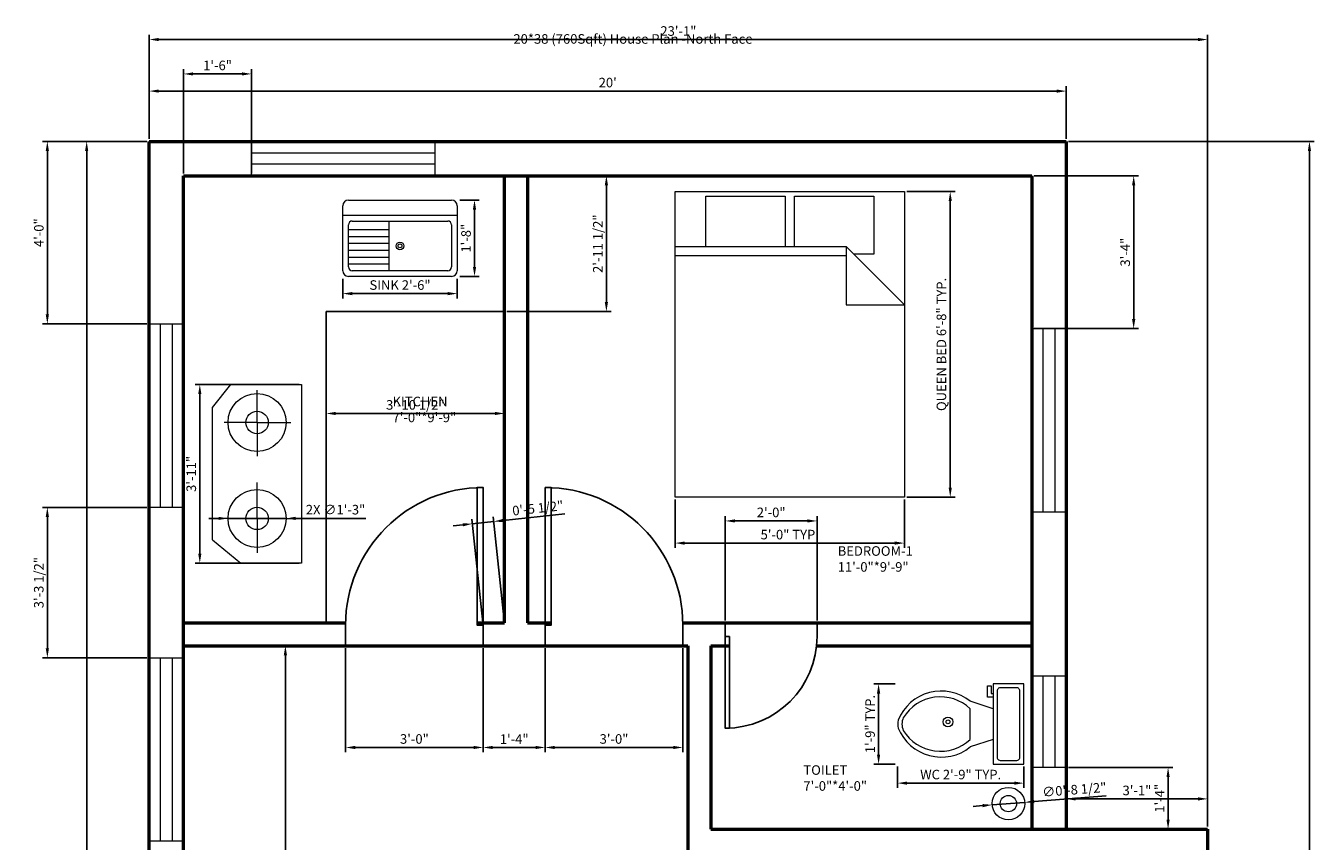
# Model space of a CAD drawing. Units: inches. Extents: x 1994 to 2331, y 1752 to 2286.
# Tile 2 of 2: x 1994 to 2331, y 2073 to 2286. Entities that reach past the tile are written whole.
import ezdxf

# ---------------------------------------------------------------- set-up
doc = ezdxf.new("R2010")
doc.units = ezdxf.units.IN
for name, color, linetype, lineweight in [('A-ANNO-DIMS', 2, 'Continuous', 18), ('A-ANNO-TEXT', 7, 'Continuous', 25), ('A-AREA-IDEN', 7, 'Continuous', 25), ('A-DOOR', 3, 'Continuous', 25), ('A-EQPM', 8, 'Continuous', 18), ('A-FLOR-CASE', 8, 'Continuous', 25), ('A-FLOR-FIXT', 8, 'Continuous', 18), ('A-FURN', 9, 'Continuous', 18), ('A-GLAZ', 4, 'Continuous', 18), ('A-WALL', 7, 'Continuous', 50)]:
    doc.layers.add(name, color=color, linetype=linetype, lineweight=lineweight)
doc.styles.get("Standard").update_dxf_attribs({"font": 'arial.ttf'})
doc.dimstyles.new('ISO-25', dxfattribs={"dimtxt": 2.5, "dimasz": 2.5, "dimexe": 1.25, "dimexo": 0.625, "dimtad": 1, "dimdec": 1, "dimlunit": 3, "dimtxsty": 'Standard', "dimcen": 2.5, "dimadec": 0, "dimazin": 0, "dimtfac": 1, "dimtdec": 1, "dimtmove": 0, "dimatfit": 3, "dimfxl": 1, "dimarcsym": 0})

# ---------------------------------------------------------------- blocks, each defined once
blk = doc.blocks.new('*U2')
for p, q in [((0, 0), (0, -6)), ((40, 0), (40, -6))]:
    blk.add_line(p, q)
blk.add_lwpolyline([(0, 0), (0, 40), (1.75, 40), (1.75, 0)], close=True)
blk.add_arc((0, 0), 40, 0, 90)
blk = doc.blocks.new('Sink-single - 30 in top')
blk.add_line((-15, -3.999996), (15, -3.999996))
for points in [[(-13.5, 0), (13.5, 0)], [(-15, -18.499996), (-15, -1.5)], [(15, -1.5), (15, -18.499996)], [(-13.5, -17.499996), (-13.5, -6.499996)], [(-12.5, -5.499996), (12.5, -5.499996)], [(13.5, -6.499996), (13.5, -17.499996)], [(13.5, -19.999996), (-13.5, -19.999996)], [(12.5, -18.499996), (-12.5, -18.499996)]]:
    blk.add_lwpolyline(points)
for radius in [1, 0.5]:
    blk.add_circle((0, -11.999996), radius)
for centre, radius, start, end in [((-13.5, -1.5), 1.5, 90, 180), ((13.5, -1.5), 1.5, 0, 90), ((-12.5, -6.499996), 1, 90, 180), ((12.5, -6.499996), 1, 0, 90), ((-13.5, -18.499996), 1.5, 180, 270), ((-12.5, -17.499996), 1, 180, 270), ((12.5, -17.499996), 1, 270, 0), ((13.5, -18.499996), 1.5, 270, 0)]:
    blk.add_arc(centre, radius, start, end)
blk = doc.blocks.new('Bed - Queen')
for p, q in [((0, -80.00003), (0, 0)), ((0, 0), (59.99999, 0)), ((59.99999, 0), (59.99999, -80.00003)), ((7.99999, -1.2), (28.79998, -1.2)), ((7.99999, -14.4), (7.99999, -1.2)), ((28.79998, -1.2), (28.79998, -14.4)), ((31.19999, -1.2), (51.99999, -1.2)), ((31.19999, -14.4), (31.19999, -1.2)), ((51.99999, -1.2), (51.99999, -16.4)), ((0, -14.4), (44.8, -14.4)), ((44.8, -16.8), (0, -16.8)), ((59.99999, -29.6), (44.8, -14.4)), ((44.8, -14.4), (44.8, -29.6)), ((51.99999, -16.4), (46.79936, -16.4)), ((44.8, -29.6), (59.99999, -29.6)), ((59.99999, -80.00003), (0, -80.00003))]:
    blk.add_line(p, q)
blk = doc.blocks.new('Toilet - top')
for p, q in [((9.5, -6), (9.5, -2)), ((-10, -8.5), (-8, -8.5)), ((-10, -9.5), (-10, -8.5)), ((-7, -9.5), (-10, -9.5)), ((-8, -8.5), (-8, -8)), ((-7, -8), (-7, -9.5)), ((-4, -8), (-6, -14)), ((4, -8), (6, -14)), ((4, -14), (-4, -14))]:
    blk.add_line(p, q)
blk.add_lwpolyline([(10.5, -8), (10.5, 0), (-10.5, 0), (-10.5, -8)], close=True)
for points in [[(-9.5, -2), (-9.5, -6)], [(8.5, -1), (-8.5, -1)], [(-8.5, -7), (8.5, -7)]]:
    blk.add_lwpolyline(points)
for centre, radius, start, end in [((-8.62, -1.88), 0.884, 81.8699, 188.1301), ((8.62, -1.88), 0.884, 351.8699, 98.1301), ((-8.62, -6.12), 0.884, 171.8699, 278.1301), ((8.62, -6.12), 0.884, 261.8699, 8.1301), ((3.52, -21.58), 12.17, 141.4691, 247.9714), ((4.2, -21.82), 11.33, 136.3677, 238.9468), ((-3.52, -21.58), 12.17, 292.0284, 38.5307), ((-4.2, -21.82), 11.33, 301.053, 43.6321), ((0, -27.88), 4, 245.7318, 294.2682), ((0, -29), 4, 254.8605, 285.1395)]:
    blk.add_arc(centre, radius, start, end)
blk = doc.blocks.new('*D6')
at = {"layer": 'A-ANNO-DIMS', "color": 0, "lineweight": -2, "transparency": 16777216}
for p, q in [((2026.58, 2256.83), (2026.58, 2270.61)), ((2029.08, 2269.36), (2264.08, 2269.36)), ((2266.58, 2256.83), (2266.58, 2270.61))]:
    blk.add_line(p, q, dxfattribs=at)
at = {"layer": 'A-ANNO-DIMS', "color": 0, "transparency": 16777216}
for points in [[(2029.08, 2269.78), (2029.08, 2268.94), (2026.58, 2269.36)], [(2264.08, 2269.78), (2264.08, 2268.94), (2266.58, 2269.36)]]:
    blk.add_solid(points, dxfattribs=at)
at = {"layer": 'Defpoints', "color": 0, "transparency": 16777216}
for p in [(2266.58, 2269.36), (2026.58, 2256.2), (2266.58, 2256.2)]:
    blk.add_point(p, dxfattribs=at)
at = {"layer": 'A-ANNO-DIMS', "color": 0, "transparency": 16777216, "insert": (2146.58, 2271.26), "char_height": 2.5, "attachment_point": 5}
blk.add_mtext("20'", dxfattribs=at)
blk = doc.blocks.new('*D7')
at = {"layer": 'A-ANNO-DIMS', "color": 0, "lineweight": -2, "transparency": 16777216}
for p, q in [((2025.95, 2256.2), (2008.97, 2256.2)), ((2010.22, 2253.7), (2010.22, 1802.7)), ((2025.95, 1800.2), (2008.97, 1800.2))]:
    blk.add_line(p, q, dxfattribs=at)
at = {"layer": 'A-ANNO-DIMS', "color": 0, "transparency": 16777216}
for points in [[(2009.8, 2253.7), (2010.63, 2253.7), (2010.22, 2256.2)], [(2009.8, 1802.7), (2010.63, 1802.7), (2010.22, 1800.2)]]:
    blk.add_solid(points, dxfattribs=at)
at = {"layer": 'Defpoints', "color": 0, "transparency": 16777216}
for p in [(2026.58, 2256.2), (2010.22, 1800.2), (2026.58, 1800.2)]:
    blk.add_point(p, dxfattribs=at)
at = {"layer": 'A-ANNO-DIMS', "color": 0, "transparency": 16777216, "insert": (2008.31, 2028.2), "char_height": 2.5, "attachment_point": 5, "rotation": 90}
blk.add_mtext("38'", dxfattribs=at)
blk = doc.blocks.new('*D8')
at = {"layer": 'A-ANNO-DIMS', "color": 0, "lineweight": -2, "transparency": 16777216}
for p, q in [((2266.58, 2076.83), (2266.58, 2085.34)), ((2269.08, 2084.09), (2301.08, 2084.09)), ((2303.58, 2076.83), (2303.58, 2085.34))]:
    blk.add_line(p, q, dxfattribs=at)
at = {"layer": 'A-ANNO-DIMS', "color": 0, "transparency": 16777216}
for points in [[(2269.08, 2084.51), (2269.08, 2083.67), (2266.58, 2084.09)], [(2301.08, 2084.51), (2301.08, 2083.67), (2303.58, 2084.09)]]:
    blk.add_solid(points, dxfattribs=at)
at = {"layer": 'Defpoints', "color": 0, "transparency": 16777216}
for p in [(2303.58, 2084.09), (2266.58, 2076.2), (2303.58, 2076.2)]:
    blk.add_point(p, dxfattribs=at)
at = {"layer": 'A-ANNO-DIMS', "color": 0, "transparency": 16777216, "insert": (2285.08, 2085.99), "char_height": 2.5, "attachment_point": 5}
blk.add_mtext('3\'-1"', dxfattribs=at)
blk = doc.blocks.new('WIN-48IN')
for p, q in [((0, 9), (48, 9)), ((0, 0), (0, 9)), ((48, 9), (48, 0)), ((0, 6), (48, 6)), ((48, 3), (0, 3)), ((48, 0), (0, 0))]:
    blk.add_line(p, q)
blk = doc.blocks.new('WIN-24IN')
for p, q in [((0, 0), (0, 24)), ((0, 24), (9, 24)), ((3, 0), (3, 24)), ((6, 24), (6, 0)), ((9, 24), (9, 0)), ((9, 0), (0, 0))]:
    blk.add_line(p, q)
blk = doc.blocks.new('*D18')
at = {"layer": 'A-ANNO-DIMS', "color": 0, "lineweight": -2, "transparency": 16777216}
for p, q in [((2224.85, 2243.05), (2237.47, 2243.05)), ((2236.22, 2165.55), (2236.22, 2240.55)), ((2224.85, 2163.05), (2237.47, 2163.05))]:
    blk.add_line(p, q, dxfattribs=at)
at = {"layer": 'A-ANNO-DIMS', "color": 0, "transparency": 16777216}
for points in [[(2235.81, 2240.55), (2236.64, 2240.55), (2236.22, 2243.05)], [(2235.81, 2165.55), (2236.64, 2165.55), (2236.22, 2163.05)]]:
    blk.add_solid(points, dxfattribs=at)
at = {"layer": 'Defpoints', "color": 0, "transparency": 16777216}
for p in [(2224.22, 2243.05), (2236.22, 2243.05), (2224.22, 2163.05)]:
    blk.add_point(p, dxfattribs=at)
at = {"layer": 'A-ANNO-DIMS', "color": 0, "transparency": 16777216, "insert": (2234.23, 2203.05), "char_height": 2.5, "attachment_point": 5, "rotation": 90}
blk.add_mtext('QUEEN BED 6\'-8" TYP.', dxfattribs=at)
blk = doc.blocks.new('*D19')
at = {"layer": 'A-ANNO-DIMS', "color": 0, "lineweight": -2, "transparency": 16777216}
for p, q in [((2164.22, 2162.43), (2164.22, 2149.8)), ((2224.22, 2162.43), (2224.22, 2149.8)), ((2166.72, 2151.05), (2221.72, 2151.05))]:
    blk.add_line(p, q, dxfattribs=at)
at = {"layer": 'A-ANNO-DIMS', "color": 0, "transparency": 16777216}
for points in [[(2166.72, 2151.47), (2166.72, 2150.63), (2164.22, 2151.05)], [(2221.72, 2151.47), (2221.72, 2150.63), (2224.22, 2151.05)]]:
    blk.add_solid(points, dxfattribs=at)
at = {"layer": 'Defpoints', "color": 0, "transparency": 16777216}
for p in [(2164.22, 2163.05), (2224.22, 2163.05), (2224.22, 2151.05)]:
    blk.add_point(p, dxfattribs=at)
at = {"layer": 'A-ANNO-DIMS', "color": 0, "transparency": 16777216, "insert": (2194.22, 2152.95), "char_height": 2.5, "attachment_point": 5}
blk.add_mtext('5\'-0" TYP.', dxfattribs=at)
blk = doc.blocks.new('*D20')
at = {"layer": 'A-ANNO-DIMS', "color": 0, "lineweight": -2, "transparency": 16777216}
for p, q in [((2222.43, 2092.55), (2222.43, 2086.97)), ((2255.47, 2092.55), (2255.47, 2086.97)), ((2224.93, 2088.22), (2252.97, 2088.22))]:
    blk.add_line(p, q, dxfattribs=at)
at = {"layer": 'A-ANNO-DIMS', "color": 0, "transparency": 16777216}
for points in [[(2224.93, 2088.64), (2224.93, 2087.8), (2222.43, 2088.22)], [(2252.97, 2088.64), (2252.97, 2087.8), (2255.47, 2088.22)]]:
    blk.add_solid(points, dxfattribs=at)
at = {"layer": 'Defpoints', "color": 0, "transparency": 16777216}
for p in [(2222.43, 2093.18), (2255.47, 2093.18), (2255.47, 2088.22)]:
    blk.add_point(p, dxfattribs=at)
at = {"layer": 'A-ANNO-DIMS', "color": 0, "transparency": 16777216, "insert": (2238.95, 2090.14), "char_height": 2.5, "attachment_point": 5}
blk.add_mtext('WC 2\'-9" TYP.', dxfattribs=at)
blk = doc.blocks.new('*D21')
at = {"layer": 'A-ANNO-DIMS', "color": 0, "lineweight": -2, "transparency": 16777216}
for p, q in [((2221.8, 2114.18), (2216.22, 2114.18)), ((2217.47, 2111.68), (2217.47, 2095.68)), ((2221.8, 2093.18), (2216.22, 2093.18))]:
    blk.add_line(p, q, dxfattribs=at)
at = {"layer": 'A-ANNO-DIMS', "color": 0, "transparency": 16777216}
for points in [[(2217.05, 2111.68), (2217.89, 2111.68), (2217.47, 2114.18)], [(2217.05, 2095.68), (2217.89, 2095.68), (2217.47, 2093.18)]]:
    blk.add_solid(points, dxfattribs=at)
at = {"layer": 'Defpoints', "color": 0, "transparency": 16777216}
for p in [(2222.43, 2114.18), (2217.47, 2093.18), (2222.43, 2093.18)]:
    blk.add_point(p, dxfattribs=at)
at = {"layer": 'A-ANNO-DIMS', "color": 0, "transparency": 16777216, "insert": (2215.57, 2103.68), "char_height": 2.5, "attachment_point": 5, "rotation": 90}
blk.add_mtext('1\'-9" TYP.', dxfattribs=at)
blk = doc.blocks.new('*D22')
at = {"layer": 'A-ANNO-DIMS', "color": 0, "lineweight": -2, "transparency": 16777216}
for p, q in [((2077.22, 2220.23), (2077.22, 2215.1)), ((2107.22, 2220.23), (2107.22, 2215.1)), ((2079.72, 2216.35), (2104.72, 2216.35))]:
    blk.add_line(p, q, dxfattribs=at)
at = {"layer": 'A-ANNO-DIMS', "color": 0, "transparency": 16777216}
for points in [[(2079.72, 2216.77), (2079.72, 2215.94), (2077.22, 2216.35)], [(2104.72, 2216.77), (2104.72, 2215.94), (2107.22, 2216.35)]]:
    blk.add_solid(points, dxfattribs=at)
at = {"layer": 'Defpoints', "color": 0, "transparency": 16777216}
for p in [(2077.22, 2220.85), (2107.22, 2220.85), (2107.22, 2216.35)]:
    blk.add_point(p, dxfattribs=at)
at = {"layer": 'A-ANNO-DIMS', "color": 0, "transparency": 16777216, "insert": (2092.22, 2218.27), "char_height": 2.5, "attachment_point": 5}
blk.add_mtext('SINK 2\'-6"', dxfattribs=at)
blk = doc.blocks.new('*D23')
at = {"layer": 'A-ANNO-DIMS', "color": 0, "lineweight": -2, "transparency": 16777216}
for p, q in [((2107.85, 2240.85), (2112.97, 2240.85)), ((2111.72, 2223.35), (2111.72, 2238.35)), ((2107.85, 2220.85), (2112.97, 2220.85))]:
    blk.add_line(p, q, dxfattribs=at)
at = {"layer": 'A-ANNO-DIMS', "color": 0, "transparency": 16777216}
for points in [[(2111.3, 2238.35), (2112.14, 2238.35), (2111.72, 2240.85)], [(2111.3, 2223.35), (2112.14, 2223.35), (2111.72, 2220.85)]]:
    blk.add_solid(points, dxfattribs=at)
at = {"layer": 'Defpoints', "color": 0, "transparency": 16777216}
for p in [(2107.22, 2240.85), (2111.72, 2240.85), (2107.22, 2220.85)]:
    blk.add_point(p, dxfattribs=at)
at = {"layer": 'A-ANNO-DIMS', "color": 0, "transparency": 16777216, "insert": (2109.82, 2230.85), "char_height": 2.5, "attachment_point": 5, "rotation": 90}
blk.add_mtext('1\'-8"', dxfattribs=at)
blk = doc.blocks.new('*D24')
at = {"layer": 'A-ANNO-DIMS', "color": 0, "lineweight": -2, "transparency": 16777216}
for p, q in [((2267.2, 2256.2), (2331.48, 2256.2)), ((2330.23, 2253.7), (2330.23, 1782.7)), ((2267.2, 1780.2), (2331.48, 1780.2))]:
    blk.add_line(p, q, dxfattribs=at)
at = {"layer": 'A-ANNO-DIMS', "color": 0, "transparency": 16777216}
for points in [[(2329.81, 2253.7), (2330.65, 2253.7), (2330.23, 2256.2)], [(2329.81, 1782.7), (2330.65, 1782.7), (2330.23, 1780.2)]]:
    blk.add_solid(points, dxfattribs=at)
at = {"layer": 'Defpoints', "color": 0, "transparency": 16777216}
for p in [(2266.58, 2256.2), (2266.58, 1780.2), (2330.23, 1780.2)]:
    blk.add_point(p, dxfattribs=at)
at = {"layer": 'A-ANNO-DIMS', "color": 0, "transparency": 16777216, "insert": (2328.33, 2018.2), "char_height": 2.5, "attachment_point": 5, "rotation": 90}
blk.add_mtext('39\'-8"', dxfattribs=at)
blk = doc.blocks.new('*D25')
at = {"layer": 'A-ANNO-DIMS', "color": 0, "lineweight": -2, "transparency": 16777216}
for p, q in [((2026.58, 2256.83), (2026.58, 2284.1)), ((2029.08, 2282.85), (2301.08, 2282.85)), ((2303.58, 2076.83), (2303.58, 2284.1))]:
    blk.add_line(p, q, dxfattribs=at)
at = {"layer": 'A-ANNO-DIMS', "color": 0, "transparency": 16777216}
for points in [[(2029.08, 2283.27), (2029.08, 2282.44), (2026.58, 2282.85)], [(2301.08, 2283.27), (2301.08, 2282.44), (2303.58, 2282.85)]]:
    blk.add_solid(points, dxfattribs=at)
at = {"layer": 'Defpoints', "color": 0, "transparency": 16777216}
for p in [(2303.58, 2282.85), (2026.58, 2256.2), (2303.58, 2076.2)]:
    blk.add_point(p, dxfattribs=at)
at = {"layer": 'A-ANNO-DIMS', "color": 0, "transparency": 16777216, "insert": (2165.08, 2284.76), "char_height": 2.5, "attachment_point": 5}
blk.add_mtext('23\'-1"', dxfattribs=at)
blk = doc.blocks.new('*D27')
at = {"layer": 'A-ANNO-DIMS', "color": 0, "lineweight": -2, "transparency": 16777216}
for p, q in [((2035.58, 2247.83), (2035.58, 2275.1)), ((2038.08, 2273.85), (2050.85, 2273.85)), ((2053.35, 2247.83), (2053.35, 2275.1))]:
    blk.add_line(p, q, dxfattribs=at)
at = {"layer": 'A-ANNO-DIMS', "color": 0, "transparency": 16777216}
for points in [[(2038.08, 2274.27), (2038.08, 2273.44), (2035.58, 2273.85)], [(2050.85, 2274.27), (2050.85, 2273.44), (2053.35, 2273.85)]]:
    blk.add_solid(points, dxfattribs=at)
at = {"layer": 'Defpoints', "color": 0, "transparency": 16777216}
for p in [(2053.35, 2273.85), (2035.58, 2247.2), (2053.35, 2247.2)]:
    blk.add_point(p, dxfattribs=at)
at = {"layer": 'A-ANNO-DIMS', "color": 0, "transparency": 16777216, "insert": (2044.47, 2275.76), "char_height": 2.5, "attachment_point": 5}
blk.add_mtext('1\'-6"', dxfattribs=at)
blk = doc.blocks.new('*D28')
at = {"layer": 'A-ANNO-DIMS', "color": 0, "lineweight": -2, "transparency": 16777216}
for p, q in [((2025.95, 2256.2), (1998.68, 2256.2)), ((1999.93, 2253.7), (1999.93, 2210.9)), ((2025.95, 2208.4), (1998.68, 2208.4))]:
    blk.add_line(p, q, dxfattribs=at)
at = {"layer": 'A-ANNO-DIMS', "color": 0, "transparency": 16777216}
for points in [[(1999.51, 2253.7), (2000.35, 2253.7), (1999.93, 2256.2)], [(1999.51, 2210.9), (2000.35, 2210.9), (1999.93, 2208.4)]]:
    blk.add_solid(points, dxfattribs=at)
at = {"layer": 'Defpoints', "color": 0, "transparency": 16777216}
for p in [(2026.58, 2256.2), (1999.93, 2208.4), (2026.58, 2208.4)]:
    blk.add_point(p, dxfattribs=at)
at = {"layer": 'A-ANNO-DIMS', "color": 0, "transparency": 16777216, "insert": (1998.03, 2232.3), "char_height": 2.5, "attachment_point": 5, "rotation": 90}
blk.add_mtext('4\'-0"', dxfattribs=at)
blk = doc.blocks.new('*D29')
at = {"layer": 'A-ANNO-DIMS', "color": 0, "lineweight": -2, "transparency": 16777216}
for p, q in [((2025.95, 2160.4), (1998.68, 2160.4)), ((1999.93, 2157.9), (1999.93, 2123.51)), ((2025.95, 2121.01), (1998.68, 2121.01))]:
    blk.add_line(p, q, dxfattribs=at)
at = {"layer": 'A-ANNO-DIMS', "color": 0, "transparency": 16777216}
for points in [[(1999.51, 2157.9), (2000.35, 2157.9), (1999.93, 2160.4)], [(1999.51, 2123.51), (2000.35, 2123.51), (1999.93, 2121.01)]]:
    blk.add_solid(points, dxfattribs=at)
at = {"layer": 'Defpoints', "color": 0, "transparency": 16777216}
for p in [(2026.58, 2160.4), (1999.93, 2121.01), (2026.58, 2121.01)]:
    blk.add_point(p, dxfattribs=at)
at = {"layer": 'A-ANNO-DIMS', "color": 0, "transparency": 16777216, "insert": (1998.01, 2140.7), "char_height": 2.5, "attachment_point": 5, "rotation": 90}
blk.add_mtext('3\'-3 1/2"', dxfattribs=at)
blk = doc.blocks.new('*D32')
at = {"layer": 'A-ANNO-DIMS', "color": 0, "lineweight": -2, "transparency": 16777216}
for p, q in [((2258.2, 2247.2), (2285.48, 2247.2)), ((2284.23, 2244.7), (2284.23, 2209.68)), ((2258.2, 2207.18), (2285.48, 2207.18))]:
    blk.add_line(p, q, dxfattribs=at)
at = {"layer": 'A-ANNO-DIMS', "color": 0, "transparency": 16777216}
for points in [[(2283.81, 2244.7), (2284.65, 2244.7), (2284.23, 2247.2)], [(2283.81, 2209.68), (2284.65, 2209.68), (2284.23, 2207.18)]]:
    blk.add_solid(points, dxfattribs=at)
at = {"layer": 'Defpoints', "color": 0, "transparency": 16777216}
for p in [(2257.58, 2247.2), (2257.58, 2207.18), (2284.23, 2207.18)]:
    blk.add_point(p, dxfattribs=at)
at = {"layer": 'A-ANNO-DIMS', "color": 0, "transparency": 16777216, "insert": (2282.33, 2227.19), "char_height": 2.5, "attachment_point": 5, "rotation": 90}
blk.add_mtext('3\'-4"', dxfattribs=at)
blk = doc.blocks.new('*D33')
at = {"layer": 'A-ANNO-DIMS', "color": 0, "lineweight": -2, "transparency": 16777216}
for p, q in [((2267.2, 2092.31), (2294.48, 2092.31)), ((2293.23, 2089.81), (2293.23, 2078.7)), ((2267.2, 2076.2), (2294.48, 2076.2))]:
    blk.add_line(p, q, dxfattribs=at)
at = {"layer": 'A-ANNO-DIMS', "color": 0, "transparency": 16777216}
for points in [[(2292.81, 2089.81), (2293.65, 2089.81), (2293.23, 2092.31)], [(2292.81, 2078.7), (2293.65, 2078.7), (2293.23, 2076.2)]]:
    blk.add_solid(points, dxfattribs=at)
at = {"layer": 'Defpoints', "color": 0, "transparency": 16777216}
for p in [(2266.58, 2092.31), (2266.58, 2076.2), (2293.23, 2076.2)]:
    blk.add_point(p, dxfattribs=at)
at = {"layer": 'A-ANNO-DIMS', "color": 0, "transparency": 16777216, "insert": (2291.35, 2084.26), "char_height": 2.5, "attachment_point": 5, "rotation": 90}
blk.add_mtext('1\'-4"', dxfattribs=at)
blk = doc.blocks.new('*D40')
at = {"layer": 'A-ANNO-DIMS', "color": 0, "lineweight": -2, "transparency": 16777216}
for p, q in [((2036.2, 2124.2), (2063.48, 2124.2)), ((2062.23, 2121.7), (2062.23, 1917.7)), ((2036.2, 1915.2), (2063.48, 1915.2))]:
    blk.add_line(p, q, dxfattribs=at)
at = {"layer": 'A-ANNO-DIMS', "color": 0, "transparency": 16777216}
for points in [[(2061.81, 2121.7), (2062.65, 2121.7), (2062.23, 2124.2)], [(2061.81, 1917.7), (2062.65, 1917.7), (2062.23, 1915.2)]]:
    blk.add_solid(points, dxfattribs=at)
at = {"layer": 'Defpoints', "color": 0, "transparency": 16777216}
for p in [(2035.58, 2124.2), (2035.58, 1915.2), (2062.23, 1915.2)]:
    blk.add_point(p, dxfattribs=at)
at = {"layer": 'A-ANNO-DIMS', "color": 0, "transparency": 16777216, "insert": (2060.33, 2019.7), "char_height": 2.5, "attachment_point": 5, "rotation": 90}
blk.add_mtext('17\'-5"', dxfattribs=at)
blk = doc.blocks.new('*D43')
at = {"layer": 'A-ANNO-DIMS', "color": 0, "lineweight": -2, "transparency": 16777216}
for p, q in [((2177.36, 2130.83), (2177.36, 2158.1)), ((2201.36, 2130.83), (2201.36, 2158.1)), ((2179.86, 2156.85), (2198.86, 2156.85))]:
    blk.add_line(p, q, dxfattribs=at)
at = {"layer": 'A-ANNO-DIMS', "color": 0, "transparency": 16777216}
for points in [[(2179.86, 2157.27), (2179.86, 2156.44), (2177.36, 2156.85)], [(2198.86, 2157.27), (2198.86, 2156.44), (2201.36, 2156.85)]]:
    blk.add_solid(points, dxfattribs=at)
at = {"layer": 'Defpoints', "color": 0, "transparency": 16777216}
for p in [(2201.36, 2156.85), (2177.36, 2130.2), (2201.36, 2130.2)]:
    blk.add_point(p, dxfattribs=at)
at = {"layer": 'A-ANNO-DIMS', "color": 0, "transparency": 16777216, "insert": (2189.36, 2158.76), "char_height": 2.5, "attachment_point": 5}
blk.add_mtext('2\'-0"', dxfattribs=at)
blk = doc.blocks.new('*D44')
at = {"layer": 'A-ANNO-DIMS', "color": 0, "lineweight": -2, "transparency": 16777216}
for p, q in [((2072.91, 2211.01), (2072.91, 2183.73)), ((2119.58, 2211.01), (2119.58, 2183.73)), ((2117.08, 2184.98), (2075.41, 2184.98))]:
    blk.add_line(p, q, dxfattribs=at)
at = {"layer": 'A-ANNO-DIMS', "color": 0, "transparency": 16777216}
for points in [[(2075.41, 2185.4), (2075.41, 2184.56), (2072.91, 2184.98)], [(2117.08, 2185.4), (2117.08, 2184.56), (2119.58, 2184.98)]]:
    blk.add_solid(points, dxfattribs=at)
at = {"layer": 'Defpoints', "color": 0, "transparency": 16777216}
for p in [(2072.91, 2211.63), (2119.58, 2211.63), (2072.91, 2184.98)]:
    blk.add_point(p, dxfattribs=at)
at = {"layer": 'A-ANNO-DIMS', "color": 0, "transparency": 16777216, "insert": (2096.24, 2186.9), "char_height": 2.5, "attachment_point": 5}
blk.add_mtext('3\'-10 1/2"', dxfattribs=at)
blk = doc.blocks.new('*D45')
at = {"layer": 'A-ANNO-DIMS', "color": 0, "lineweight": -2, "transparency": 16777216}
for p, q in [((2120.2, 2247.2), (2147.48, 2247.2)), ((2146.23, 2244.7), (2146.23, 2214.13)), ((2120.2, 2211.63), (2147.48, 2211.63))]:
    blk.add_line(p, q, dxfattribs=at)
at = {"layer": 'A-ANNO-DIMS', "color": 0, "transparency": 16777216}
for points in [[(2145.81, 2244.7), (2146.65, 2244.7), (2146.23, 2247.2)], [(2145.81, 2214.13), (2146.65, 2214.13), (2146.23, 2211.63)]]:
    blk.add_solid(points, dxfattribs=at)
at = {"layer": 'Defpoints', "color": 0, "transparency": 16777216}
for p in [(2119.58, 2247.2), (2119.58, 2211.63), (2146.23, 2211.63)]:
    blk.add_point(p, dxfattribs=at)
at = {"layer": 'A-ANNO-DIMS', "color": 0, "transparency": 16777216, "insert": (2144.31, 2229.42), "char_height": 2.5, "attachment_point": 5, "rotation": 90}
blk.add_mtext('2\'-11 1/2"', dxfattribs=at)
blk = doc.blocks.new('*D50')
at = {"layer": 'A-ANNO-DIMS', "color": 0, "lineweight": -2, "transparency": 16777216}
for p, q in [((2119.22, 2156.97), (2135.35, 2158.7)), ((2108.66, 2155.84), (2106.17, 2155.57)), ((2113.92, 2130.23), (2111.01, 2157.35)), ((2111.14, 2156.1), (2116.74, 2156.7)), ((2119.51, 2130.83), (2116.6, 2157.95))]:
    blk.add_line(p, q, dxfattribs=at)
at = {"layer": 'A-ANNO-DIMS', "color": 0, "transparency": 16777216}
for points in [[(2108.61, 2156.25), (2108.7, 2155.42), (2111.14, 2156.1)], [(2119.18, 2157.38), (2119.27, 2156.55), (2116.74, 2156.7)]]:
    blk.add_solid(points, dxfattribs=at)
at = {"layer": 'Defpoints', "color": 0, "transparency": 16777216}
for p in [(2116.74, 2156.7), (2113.99, 2129.6), (2119.58, 2130.2)]:
    blk.add_point(p, dxfattribs=at)
at = {"layer": 'A-ANNO-DIMS', "color": 0, "transparency": 16777216, "insert": (2128.32, 2159.87), "char_height": 2.5, "attachment_point": 5, "rotation": 6.1252}
blk.add_mtext('0\'-5 1/2"', dxfattribs=at)
blk = doc.blocks.new('*D51')
at = {"layer": 'A-ANNO-DIMS', "color": 0, "lineweight": -2, "transparency": 16777216}
for p, q in [((2077.99, 2123.58), (2077.99, 2096.3)), ((2113.99, 2123.58), (2113.99, 2096.3)), ((2111.49, 2097.55), (2080.49, 2097.55))]:
    blk.add_line(p, q, dxfattribs=at)
at = {"layer": 'A-ANNO-DIMS', "color": 0, "transparency": 16777216}
for points in [[(2080.49, 2097.97), (2080.49, 2097.14), (2077.99, 2097.55)], [(2111.49, 2097.97), (2111.49, 2097.14), (2113.99, 2097.55)]]:
    blk.add_solid(points, dxfattribs=at)
at = {"layer": 'Defpoints', "color": 0, "transparency": 16777216}
for p in [(2077.99, 2124.2), (2113.99, 2124.2), (2077.99, 2097.55)]:
    blk.add_point(p, dxfattribs=at)
at = {"layer": 'A-ANNO-DIMS', "color": 0, "transparency": 16777216, "insert": (2095.99, 2099.46), "char_height": 2.5, "attachment_point": 5}
blk.add_mtext('3\'-0"', dxfattribs=at)
blk = doc.blocks.new('*D52')
at = {"layer": 'A-ANNO-DIMS', "color": 0, "lineweight": -2, "transparency": 16777216}
for p, q in [((2113.99, 2123.58), (2113.99, 2096.3)), ((2130.23, 2123.58), (2130.23, 2096.3)), ((2127.73, 2097.55), (2116.49, 2097.55))]:
    blk.add_line(p, q, dxfattribs=at)
at = {"layer": 'A-ANNO-DIMS', "color": 0, "transparency": 16777216}
for points in [[(2116.49, 2097.97), (2116.49, 2097.14), (2113.99, 2097.55)], [(2127.73, 2097.97), (2127.73, 2097.14), (2130.23, 2097.55)]]:
    blk.add_solid(points, dxfattribs=at)
at = {"layer": 'Defpoints', "color": 0, "transparency": 16777216}
for p in [(2113.99, 2124.2), (2130.23, 2124.2), (2113.99, 2097.55)]:
    blk.add_point(p, dxfattribs=at)
at = {"layer": 'A-ANNO-DIMS', "color": 0, "transparency": 16777216, "insert": (2122.11, 2099.43), "char_height": 2.5, "attachment_point": 5}
blk.add_mtext('1\'-4"', dxfattribs=at)
blk = doc.blocks.new('*D53')
at = {"layer": 'A-ANNO-DIMS', "color": 0, "lineweight": -2, "transparency": 16777216}
for p, q in [((2130.23, 2123.58), (2130.23, 2096.3)), ((2166.23, 2123.58), (2166.23, 2096.3)), ((2163.73, 2097.55), (2132.73, 2097.55))]:
    blk.add_line(p, q, dxfattribs=at)
at = {"layer": 'A-ANNO-DIMS', "color": 0, "transparency": 16777216}
for points in [[(2132.73, 2097.97), (2132.73, 2097.14), (2130.23, 2097.55)], [(2163.73, 2097.97), (2163.73, 2097.14), (2166.23, 2097.55)]]:
    blk.add_solid(points, dxfattribs=at)
at = {"layer": 'Defpoints', "color": 0, "transparency": 16777216}
for p in [(2130.23, 2124.2), (2166.23, 2124.2), (2130.23, 2097.55)]:
    blk.add_point(p, dxfattribs=at)
at = {"layer": 'A-ANNO-DIMS', "color": 0, "transparency": 16777216, "insert": (2148.23, 2099.46), "char_height": 2.5, "attachment_point": 5}
blk.add_mtext('3\'-0"', dxfattribs=at)
blk = doc.blocks.new('*D54')
at = {"layer": 'A-ANNO-DIMS', "color": 0, "lineweight": -2, "transparency": 16777216}
for p, q in [((2065.85, 2192.56), (2038.58, 2192.56)), ((2039.83, 2148.27), (2039.83, 2190.06)), ((2065.85, 2145.77), (2038.58, 2145.77))]:
    blk.add_line(p, q, dxfattribs=at)
at = {"layer": 'A-ANNO-DIMS', "color": 0, "transparency": 16777216}
for points in [[(2039.41, 2190.06), (2040.24, 2190.06), (2039.83, 2192.56)], [(2039.41, 2148.27), (2040.24, 2148.27), (2039.83, 2145.77)]]:
    blk.add_solid(points, dxfattribs=at)
at = {"layer": 'Defpoints', "color": 0, "transparency": 16777216}
for p in [(2039.83, 2192.56), (2066.48, 2192.56), (2066.48, 2145.77)]:
    blk.add_point(p, dxfattribs=at)
at = {"layer": 'A-ANNO-DIMS', "color": 0, "transparency": 16777216, "insert": (2037.92, 2169.16), "char_height": 2.5, "attachment_point": 5, "rotation": 90}
blk.add_mtext('3\'-11"', dxfattribs=at)
blk = doc.blocks.new('*D55')
at = {"layer": 'A-ANNO-DIMS', "color": 0, "lineweight": -2, "transparency": 16777216}
for p, q in [((2044.73, 2157.51), (2042.23, 2157.51)), ((2047.23, 2157.51), (2062.4, 2157.51)), ((2083.3, 2157.51), (2064.9, 2157.51))]:
    blk.add_line(p, q, dxfattribs=at)
at = {"layer": 'A-ANNO-DIMS', "color": 0, "transparency": 16777216}
for points in [[(2044.73, 2157.93), (2044.73, 2157.1), (2047.23, 2157.51)], [(2064.9, 2157.93), (2064.9, 2157.1), (2062.4, 2157.51)]]:
    blk.add_solid(points, dxfattribs=at)
at = {"layer": 'Defpoints', "color": 0, "transparency": 16777216}
for p in [(2047.23, 2157.51), (2062.4, 2157.51)]:
    blk.add_point(p, dxfattribs=at)
at = {"layer": 'A-ANNO-DIMS', "color": 0, "transparency": 16777216, "insert": (2075.35, 2159.48), "char_height": 2.5, "attachment_point": 5, "rotation": 359.9982}
blk.add_mtext('2X ∅1\'-3"', dxfattribs=at)
blk = doc.blocks.new('*D57')
at = {"layer": 'A-ANNO-DIMS', "color": 0, "lineweight": -2, "transparency": 16777216}
for p, q in [((2277.07, 2084.86), (2258.19, 2083.39)), ((2244.7, 2082.33), (2242.21, 2082.14)), ((2247.19, 2082.53), (2255.69, 2083.19))]:
    blk.add_line(p, q, dxfattribs=at)
at = {"layer": 'A-ANNO-DIMS', "color": 0, "transparency": 16777216}
for points in [[(2244.67, 2082.75), (2244.73, 2081.92), (2247.19, 2082.53)], [(2258.15, 2083.8), (2258.22, 2082.97), (2255.69, 2083.19)]]:
    blk.add_solid(points, dxfattribs=at)
at = {"layer": 'Defpoints', "color": 0, "transparency": 16777216}
for p in [(2247.19, 2082.53), (2255.69, 2083.19)]:
    blk.add_point(p, dxfattribs=at)
at = {"layer": 'A-ANNO-DIMS', "color": 0, "transparency": 16777216, "insert": (2268.72, 2086.19), "char_height": 2.5, "attachment_point": 5, "rotation": 4.4611}
blk.add_mtext('∅0\'-8 1/2"', dxfattribs=at)

msp = doc.modelspace()

# ---------------------------------------------------------------- linework, layer by layer
at = {"layer": 'A-EQPM'}
for p, q in [((2043.15, 2186.58), (2047.99, 2192.56)), ((2054.81, 2182.62), (2054.81, 2191.11)), ((2054.81, 2182.62), (2046.18, 2182.62)), ((2054.81, 2182.62), (2063.67, 2182.62)), ((2054.81, 2182.62), (2054.81, 2173.81)), ((2054.81, 2157.51), (2054.81, 2166.89)), ((2054.81, 2157.51), (2045.66, 2157.51)), ((2054.81, 2157.51), (2064.32, 2157.51)), ((2054.81, 2157.51), (2054.81, 2148.48)), ((2043.15, 2151.94), (2050.59, 2145.77))]:
    msp.add_line(p, q, dxfattribs=at)
for points in [[(2047.99, 2192.56), (2066.48, 2192.56), (2066.48, 2145.77), (2050.59, 2145.77)], [(2043.15, 2151.94), (2043.15, 2186.58)]]:
    msp.add_lwpolyline(points, dxfattribs=at)
for centre, radius in [((2054.81, 2182.62), 7.59), ((2054.81, 2182.62), 2.94), ((2054.81, 2157.51), 7.59), ((2054.81, 2157.51), 2.94)]:
    msp.add_circle(centre, radius, dxfattribs=at)
at = {"layer": 'A-FLOR-CASE'}
for p, q in [((2072.91, 2130.2), (2072.91, 2211.63)), ((2072.91, 2211.63), (2119.58, 2211.63))]:
    msp.add_line(p, q, dxfattribs=at)
at = {"layer": 'A-FLOR-FIXT'}
for p, q in [((2078.72, 2233.13), (2089.28, 2233.13)), ((2089.28, 2235.35), (2089.28, 2222.35)), ((2078.72, 2231.33), (2089.28, 2231.33)), ((2078.72, 2229.53), (2089.28, 2229.53)), ((2078.72, 2227.73), (2089.28, 2227.73)), ((2078.72, 2225.93), (2089.28, 2225.93)), ((2078.72, 2224.13), (2089.28, 2224.13))]:
    msp.add_line(p, q, dxfattribs=at)
for centre, radius in [((2235.63, 2104.25), 1.28), ((2235.63, 2104.25), 0.503), ((2251.44, 2082.86), 4.26), ((2251.44, 2082.86), 2.13)]:
    msp.add_circle(centre, radius, dxfattribs=at)
at = {"layer": 'A-WALL'}
for p, q in [((2026.58, 2256.2), (2266.58, 2256.2)), ((2026.58, 1800.2), (2026.58, 2256.2)), ((2266.58, 2256.2), (2266.58, 2076.2)), ((2035.58, 2247.2), (2257.58, 2247.2)), ((2035.58, 1809.2), (2035.58, 2247.2)), ((2119.58, 2130.2), (2119.58, 2247.2)), ((2125.58, 2247.2), (2125.58, 2130.2)), ((2257.58, 2247.2), (2257.58, 2076.2)), ((2035.58, 2130.2), (2077.99, 2130.2)), ((2112.41, 2130.2), (2119.58, 2130.2)), ((2125.58, 2130.2), (2131.81, 2130.2)), ((2166.23, 2130.2), (2257.58, 2130.2)), ((2035.58, 2124.2), (2167.58, 2124.2)), ((2167.58, 2124.2), (2167.58, 2070.2)), ((2173.58, 2124.2), (2173.58, 2076.2)), ((2173.58, 2124.2), (2178.41, 2124.2)), ((2201.24, 2124.2), (2257.58, 2124.2)), ((2173.58, 2076.2), (2266.58, 2076.2)), ((2266.58, 2076.2), (2303.58, 2076.2)), ((2303.58, 2076.2), (2303.58, 1980.2))]:
    msp.add_line(p, q, dxfattribs=at)

# ---------------------------------------------------------------- block references
at = {"layer": 'A-DOOR', "yscale": 0.8999999999998362, "zscale": 0.8999999999998362}
for p, xscale in [((2113.99, 2129.6), -0.8999999999998362), ((2130.23, 2129.6), 0.8999999999998362)]:
    msp.add_blockref('*U2', p, dxfattribs=dict(at, xscale=xscale))
at = {"layer": 'A-DOOR', "xscale": -0.5999999999999969, "yscale": 0.5999999999999969, "zscale": 0.5999999999999969, "rotation": 180}
msp.add_blockref('*U2', (2177.36, 2126.6), dxfattribs=at)
at = {"layer": 'A-FLOR-FIXT'}
msp.add_blockref('Sink-single - 30 in top', (2092.22, 2240.85), dxfattribs=at)
at = {"layer": 'A-FLOR-FIXT', "rotation": 270}
msp.add_blockref('Toilet - top', (2255.47, 2103.68), dxfattribs=at)
at = {"layer": 'A-FURN'}
msp.add_blockref('Bed - Queen', (2164.22, 2243.05), dxfattribs=at)
at = {"layer": 'A-GLAZ'}
for name, p in [('WIN-48IN', (2053.35, 2247.2)), ('WIN-24IN', (2257.58, 2092.31))]:
    msp.add_blockref(name, p, dxfattribs=at)
for p, rotation in [((2026.58, 2208.4), 269.9999999999998), ((2257.58, 2207.18), 270.0000000000021), ((2026.58, 2121.01), 270.0000000000002)]:
    msp.add_blockref('WIN-48IN', p, dxfattribs=dict(at, rotation=rotation))

# ---------------------------------------------------------------- texts
at = {"layer": 'A-ANNO-TEXT', "insert": (2121.9, 2284.26), "char_height": 2.5, "attachment_point": 1}
msp.add_mtext_dynamic_manual_height_columns('20*38 (760Sqft) House Plan -North Face', width=234.8436, gutter_width=12.5, heights=[0], dxfattribs=at)
at = {"layer": 'A-AREA-IDEN', "char_height": 2.5, "attachment_point": 1}
for s, width, insert in [('KITCHEN\\P7\'-0"*9\'-9"', 33.3176, (2090.27, 2189.36)), ('BEDROOM-1\\P11\'-0"*9\'-9"', 53.0926, (2206.77, 2150.23)), ('TOILET\\P7\'-0"*4\'-0"', 39.0756, (2197.79, 2092.9))]:
    msp.add_mtext_dynamic_manual_height_columns(s, width=width, gutter_width=12.5, heights=[0], dxfattribs=dict(at, insert=insert))

# ---------------------------------------------------------------- dimensions: what is measured, and where the dimension line sits
at = {"layer": 'A-ANNO-DIMS'}
for base, p1, p2, override, picture, middle in [((2303.58, 2282.85), (2026.58, 2256.2), (2303.58, 2076.2), {"dimdec": 1, "dimlfac": 1, "dimrnd": 0, "dimzin": 1, "dimdsep": 46, "dimlunit": 4, "dimfrac": 2}, '*D25', (2165.08, 2284.76)), ((2053.35, 2273.85), (2035.58, 2247.2), (2053.35, 2247.2), {"dimdec": 1, "dimlfac": 1, "dimrnd": 0, "dimzin": 1, "dimdsep": 46, "dimlunit": 4, "dimfrac": 2}, '*D27', (2044.47, 2275.76)), ((2266.58, 2269.36), (2026.58, 2256.2), (2266.58, 2256.2), {"dimclrd": 0, "dimclre": 0, "dimclrt": 0}, '*D6', (2146.58, 2271.26)), ((2201.36, 2156.85), (2177.36, 2130.2), (2201.36, 2130.2), {"dimdec": 1, "dimlfac": 1, "dimrnd": 0, "dimzin": 1, "dimdsep": 46, "dimlunit": 4, "dimfrac": 2}, '*D43', (2189.36, 2158.76)), ((2303.58, 2084.09), (2266.58, 2076.2), (2303.58, 2076.2), {"dimclrd": 0, "dimclre": 0, "dimclrt": 0}, '*D8', (2285.08, 2085.99))]:
    dim = msp.add_linear_dim(base=base, p1=p1, p2=p2, dimstyle='ISO-25', override=override, dxfattribs=at)
    dim.commit()
    dim.dimension.update_dxf_attribs({"geometry": picture, "text_midpoint": middle})
for base, p1, p2, angle, override, picture, middle in [((1999.93, 2208.4), (2026.58, 2256.2), (2026.58, 2208.4), 90, {"dimdec": 1, "dimlfac": 1, "dimrnd": 0, "dimzin": 1, "dimdsep": 46, "dimlunit": 4, "dimfrac": 2}, '*D28', (1998.03, 2232.3)), ((2010.22, 1800.2), (2026.58, 2256.2), (2026.58, 1800.2), 90, {"dimclrd": 0, "dimclre": 0, "dimclrt": 0}, '*D7', (2008.31, 2028.2)), ((2330.23, 1780.2), (2266.58, 2256.2), (2266.58, 1780.2), 90, {"dimdec": 1, "dimlfac": 1, "dimrnd": 0, "dimzin": 1, "dimdsep": 46, "dimlunit": 4, "dimfrac": 2}, '*D24', (2328.33, 2018.2)), ((2146.23, 2211.63), (2119.58, 2247.2), (2119.58, 2211.63), 270, {"dimdec": 1, "dimlfac": 1, "dimrnd": 0, "dimzin": 1, "dimdsep": 46, "dimlunit": 4, "dimfrac": 2}, '*D45', (2144.31, 2229.42)), ((2284.23, 2207.18), (2257.58, 2247.2), (2257.58, 2207.18), 270, {"dimdec": 1, "dimlfac": 1, "dimrnd": 0, "dimzin": 1, "dimdsep": 46, "dimlunit": 4, "dimfrac": 2}, '*D32', (2282.33, 2227.19)), ((2111.72, 2240.85), (2107.22, 2220.85), (2107.22, 2240.85), 90, {"dimdec": 1, "dimlfac": 1, "dimrnd": 0, "dimzin": 1, "dimdsep": 46, "dimlunit": 4, "dimfrac": 2}, '*D23', (2109.82, 2230.85)), ((2072.91, 2184.98), (2119.58, 2211.63), (2072.91, 2211.63), 180, {"dimdec": 1, "dimlfac": 1, "dimrnd": 0, "dimzin": 1, "dimdsep": 46, "dimlunit": 4, "dimfrac": 2}, '*D44', (2096.24, 2186.9)), ((2039.83, 2192.56), (2066.48, 2145.77), (2066.48, 2192.56), 90, {"dimdec": 1, "dimlfac": 1, "dimrnd": 0, "dimzin": 1, "dimdsep": 46, "dimlunit": 4, "dimfrac": 2}, '*D54', (2037.92, 2169.16)), ((2116.74, 2156.7), (2113.99, 2129.6), (2119.58, 2130.2), 6.1252, {"dimdec": 1, "dimlfac": 1, "dimrnd": 0, "dimzin": 1, "dimdsep": 46, "dimlunit": 4, "dimfrac": 2}, '*D50', (2128.32, 2159.87)), ((1999.93, 2121.01), (2026.58, 2160.4), (2026.58, 2121.01), 90, {"dimdec": 1, "dimlfac": 1, "dimrnd": 0, "dimzin": 1, "dimdsep": 46, "dimlunit": 4, "dimfrac": 2}, '*D29', (1998.01, 2140.7)), ((2062.23, 1915.2), (2035.58, 2124.2), (2035.58, 1915.2), 270, {"dimdec": 1, "dimlfac": 1, "dimrnd": 0, "dimzin": 1, "dimdsep": 46, "dimlunit": 4, "dimfrac": 2}, '*D40', (2060.33, 2019.7)), ((2077.99, 2097.55), (2113.99, 2124.2), (2077.99, 2124.2), 180, {"dimdec": 1, "dimlfac": 1, "dimrnd": 0, "dimzin": 1, "dimdsep": 46, "dimlunit": 4, "dimfrac": 2}, '*D51', (2095.99, 2099.46)), ((2113.99, 2097.55), (2130.23, 2124.2), (2113.99, 2124.2), 180, {"dimdec": 1, "dimlfac": 1, "dimrnd": 0, "dimzin": 1, "dimdsep": 46, "dimlunit": 4, "dimfrac": 2}, '*D52', (2122.11, 2099.43)), ((2130.23, 2097.55), (2166.23, 2124.2), (2130.23, 2124.2), 180, {"dimdec": 1, "dimlfac": 1, "dimrnd": 0, "dimzin": 1, "dimdsep": 46, "dimlunit": 4, "dimfrac": 2}, '*D53', (2148.23, 2099.46)), ((2293.23, 2076.2), (2266.58, 2092.31), (2266.58, 2076.2), 270, {"dimdec": 1, "dimlfac": 1, "dimrnd": 0, "dimzin": 1, "dimdsep": 46, "dimlunit": 4, "dimfrac": 2}, '*D33', (2291.35, 2084.26))]:
    dim = msp.add_linear_dim(base=base, p1=p1, p2=p2, angle=angle, dimstyle='ISO-25', override=override, dxfattribs=at)
    dim.commit()
    dim.dimension.update_dxf_attribs({"geometry": picture, "text_midpoint": middle})
for base, p1, p2, angle, text, picture, middle in [((2236.22, 2243.05), (2224.22, 2163.05), (2224.22, 2243.05), 90, 'QUEEN BED <> TYP.', '*D18', (2234.23, 2203.05)), ((2217.47, 2093.18), (2222.43, 2114.18), (2222.43, 2093.18), 270, '<> TYP.', '*D21', (2215.57, 2103.68))]:
    dim = msp.add_linear_dim(base=base, p1=p1, p2=p2, angle=angle, text=text, dimstyle='ISO-25', override={"dimdec": 1, "dimlfac": 1, "dimrnd": 0, "dimzin": 1, "dimdsep": 46, "dimlunit": 4, "dimfrac": 2}, dxfattribs=at)
    dim.commit()
    dim.dimension.update_dxf_attribs({"geometry": picture, "text_midpoint": middle})
for base, p1, p2, text, picture, middle in [((2107.22, 2216.35), (2077.22, 2220.85), (2107.22, 2220.85), 'SINK <>', '*D22', (2092.22, 2218.27)), ((2224.22, 2151.05), (2164.22, 2163.05), (2224.22, 2163.05), '<> TYP.', '*D19', (2194.22, 2152.95)), ((2255.47, 2088.22), (2222.43, 2093.18), (2255.47, 2093.18), 'WC <> TYP.', '*D20', (2238.95, 2090.14))]:
    dim = msp.add_linear_dim(base=base, p1=p1, p2=p2, text=text, dimstyle='ISO-25', override={"dimdec": 1, "dimlfac": 1, "dimrnd": 0, "dimzin": 1, "dimdsep": 46, "dimlunit": 4, "dimfrac": 2}, dxfattribs=at)
    dim.commit()
    dim.dimension.update_dxf_attribs({"geometry": picture, "text_midpoint": middle})
dim = msp.add_diameter_dim_2p(p1=(2047.23, 2157.51), p2=(2062.4, 2157.51), text='2X <>', dimstyle='ISO-25', override={"dimdec": 1, "dimlfac": 1, "dimrnd": 0, "dimzin": 1, "dimdsep": 46, "dimlunit": 4, "dimfrac": 2}, dxfattribs=at)
dim.commit()
dim.dimension.update_dxf_attribs({"geometry": '*D55', "text_midpoint": (2075.35, 2157.51)})
dim = msp.add_diameter_dim_2p(p1=(2247.19, 2082.53), p2=(2255.69, 2083.19), dimstyle='ISO-25', override={"dimdec": 1, "dimlfac": 1, "dimrnd": 0, "dimzin": 1, "dimdsep": 46, "dimlunit": 4, "dimfrac": 2}, dxfattribs=at)
dim.commit()
dim.dimension.update_dxf_attribs({"geometry": '*D57', "text_midpoint": (2268.87, 2084.22), "dimtype": 163})

doc.saveas('drawing.dxf')
